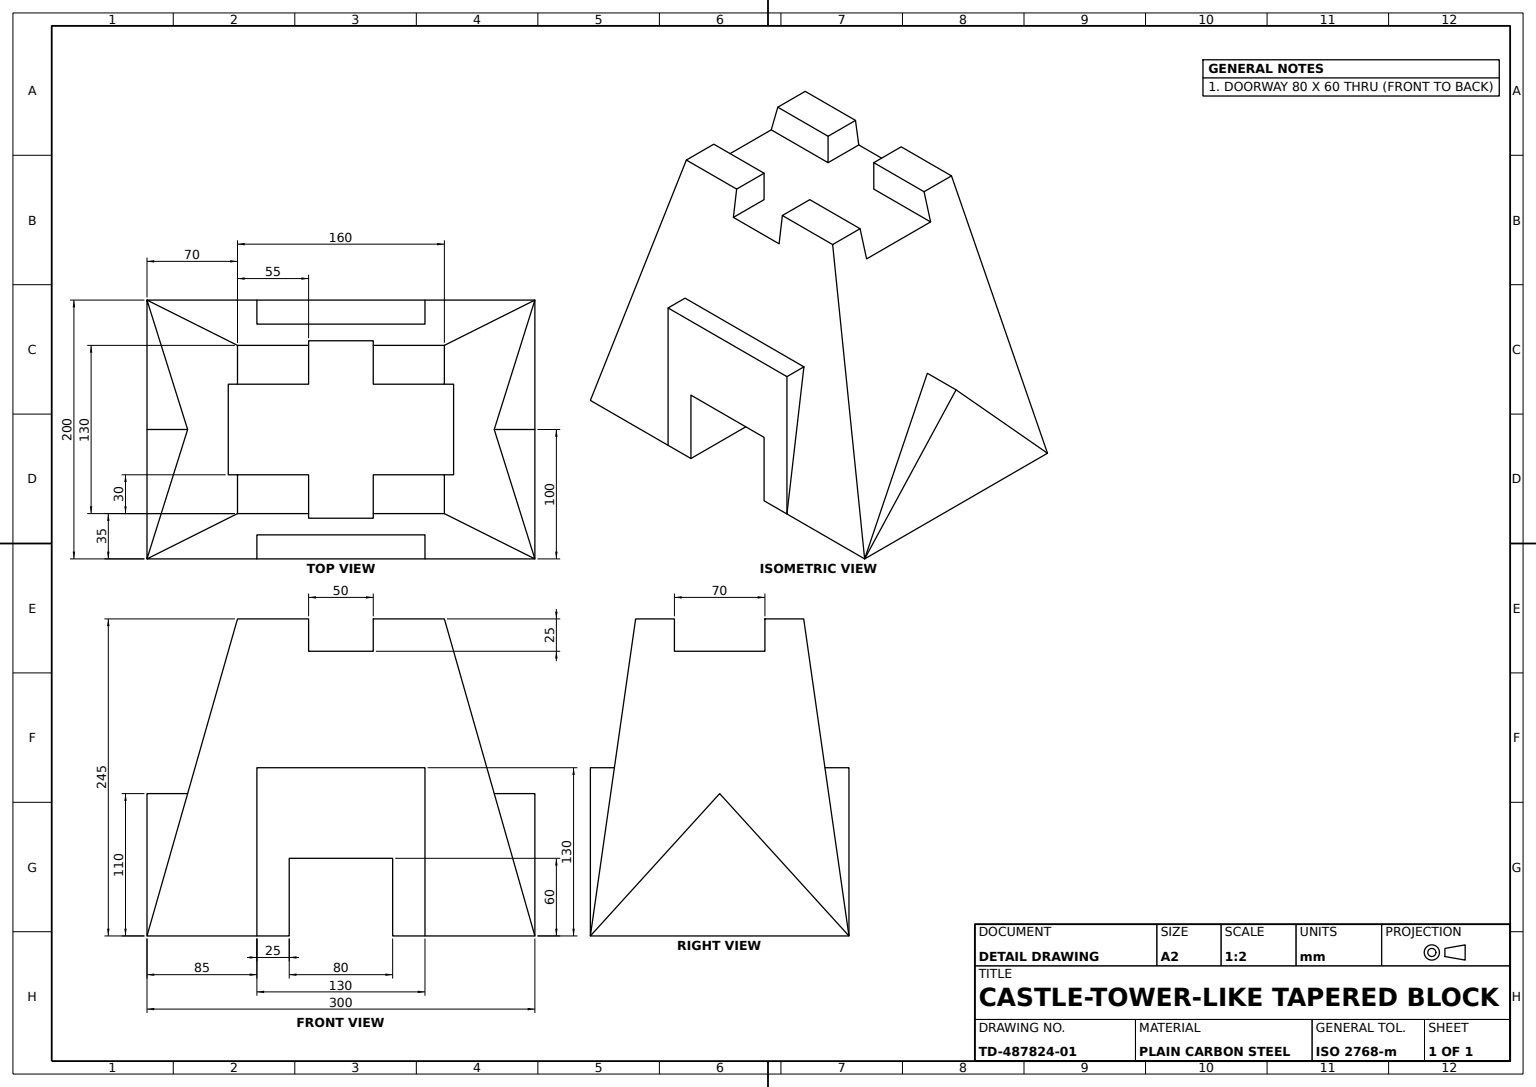
from build123d import *

# Parameters (mm, degrees)
GATE_BLOCK_PROFILE_130X130_W   = 130
GATE_BLOCK_PROFILE_130X130_H   = 130
GATE_BLOCK_DEPTH               = 100
SIDE_BUTTRESS_DEPTH            = 150
DOORWAY_CUT_DEPTH              = 305.179223648
DOORWAY_CUT_DEPTH_BACK         = 305.179223648
DOORWAY_PROFILE_60X80_W        = 80
DOORWAY_PROFILE_60X80_H        = 60
CRENELLATION_CUT_25_DEEP_DEPTH = 25


with BuildPart() as part:
    # Top Profile 160x130 → Pyramidal Body Loft section 0
    with BuildSketch(Plane(origin=(0, 245, 0), x_dir=(1, 0, 0), z_dir=(0, 1, 0))):
        with BuildLine():
            Line((-80, -65), (80, -65))
            Line((80, -65), (80, 65))
            Line((80, 65), (-80, 65))
            Line((-80, 65), (-80, -65))
        make_face()
    # Base Profile 300x200 → Pyramidal Body Loft section 1
    with BuildSketch(Plane(origin=(0, 0, 0), x_dir=(1, 0, 0), z_dir=(0, 1, 0))):
        with BuildLine():
            Line((-150, -100), (150, -100))
            Line((150, -100), (150, 100))
            Line((150, 100), (-150, 100))
            Line((-150, 100), (-150, -100))
        make_face()
    loft()

    # Gate Block Profile 130x130 → Gate Block (add, symmetric)
    with BuildSketch(Plane.XY):
        with Locations((0, 65)):
            Rectangle(GATE_BLOCK_PROFILE_130X130_W, GATE_BLOCK_PROFILE_130X130_H)
    extrude(amount=GATE_BLOCK_DEPTH, both=True)

    # Side Buttress Profile → Side Buttress (add, symmetric)
    with BuildSketch(Plane(origin=(0, 0, 0), x_dir=(0, 0, -1), z_dir=(1, 0, 0))):
        Polygon((-100, 0), (0, 110), (100, 0), align=None)
    extrude(amount=SIDE_BUTTRESS_DEPTH, both=True)

    # Doorway Profile 60x80 → Doorway Cut (cut, two sides: drawn at the far end of the back side and taken through both)
    with BuildSketch(Plane.XY.offset(-DOORWAY_CUT_DEPTH_BACK)):
        with Locations((0, 30)):
            Rectangle(DOORWAY_PROFILE_60X80_W, DOORWAY_PROFILE_60X80_H)
    extrude(amount=DOORWAY_CUT_DEPTH + DOORWAY_CUT_DEPTH_BACK, mode=Mode.SUBTRACT)

    # Crenellation Profile → Crenellation Cut 25 Deep (cut)
    with BuildSketch(Plane(origin=(0, 245, 0), x_dir=(1, 0, 0), z_dir=(0, 1, 0))):
        Polygon((-25, 65), (-25, 35), (-80, 35), (-93.798877222, 35), (-93.798877222, -35), (-80, -35), (-25, -35), (-25, -65), (-25, -87.972860003), (25, -87.972860003), (25, -65), (25, -35), (80, -35), (94.18727837, -35), (94.18727837, 35), (80, 35), (25, 35), (25, 65), (25, 74.605387162), (-25, 74.605387162), align=None)
    extrude(amount=-CRENELLATION_CUT_25_DEEP_DEPTH, mode=Mode.SUBTRACT)


solid = part.part
